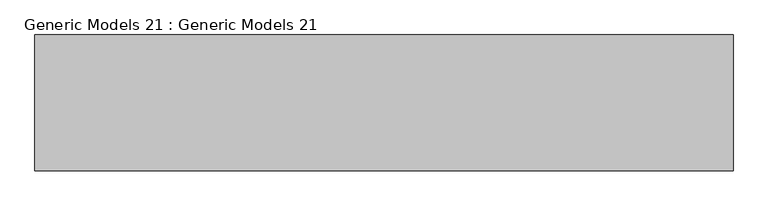
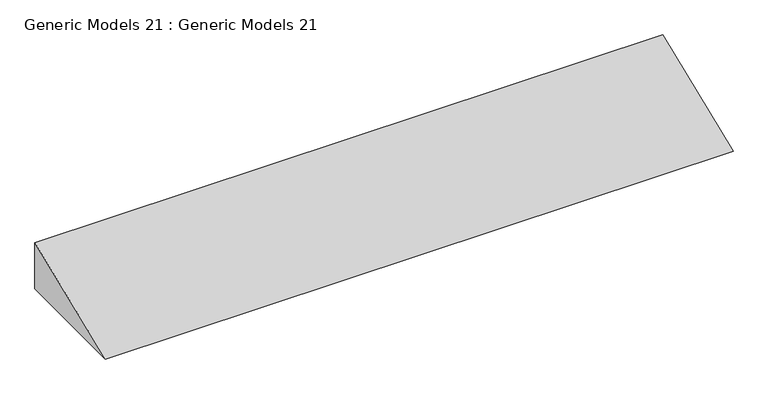
"""IFC4 building model written with IfcOpenShell, lengths in millimetres: proxy geometry, Generic Models 21 : Generic Models 21."""

from ifc_helpers import new_model, si_unit, frame, origin, place, context, project, spatial, polyline, outline, extrude, source, transform, mapped, element, save


def generic_models_21_generic_models_21_217a5a39(model_context):
    return source(origin(), model_context, "Body", "SweptSolid", [
        extrude(outline(polyline([(-9574.3210084, 0.0), (-10082.3210084, 0.0), (-10336.3210084, 0.0), (-9574.3210084, 304.8), (-9574.3210084, 0.0)])), frame((-6319.9330789, 0.0, 0.0), z_axis=(1.0, 0.0, 0.0), x_axis=(0.0, 1.0, 0.0)), (0.0, 0.0, 1.0), 3913.172335),
    ])


if __name__ == "__main__":
    model = new_model("IFC4")
    model_context = context("Model", 3, world=origin())
    ifc_project = project(units=[si_unit("LENGTHUNIT", "METRE", prefix="MILLI")], contexts=[model_context])
    site = spatial("IfcSite", under=ifc_project)
    building = spatial("IfcBuilding", under=site)
    placement = place(None, origin())
    generic_models_21_generic_models_21_shape = generic_models_21_generic_models_21_217a5a39(model_context)
    element("IfcBuildingElementProxy", 1, Name="Generic Models 21 : Generic Models 21", ObjectType="Generic Models 21 : Generic Models 21", at=placement, inside=building, context=model_context, shape_type="MappedRepresentation", body=[
        mapped(generic_models_21_generic_models_21_shape, transform((0.0, 0.0, 0.0), x_axis=(1.0, 0.0, 0.0), y_axis=(0.0, 1.0, 0.0), z_axis=(0.0, 0.0, 1.0))),
    ])
    save(model, "model.ifc")

# Revit data of these elements
# Element 1 (IfcBuildingElementProxy, "Generic Models 21 : Generic Models 21")
#   Materials on its faces: "CAST IN PLACE STAIRS"
# Materials
#   "CAST IN PLACE STAIRS": class "Generic", colour RGB 120 120 120, transparency 0, Cost = 0
